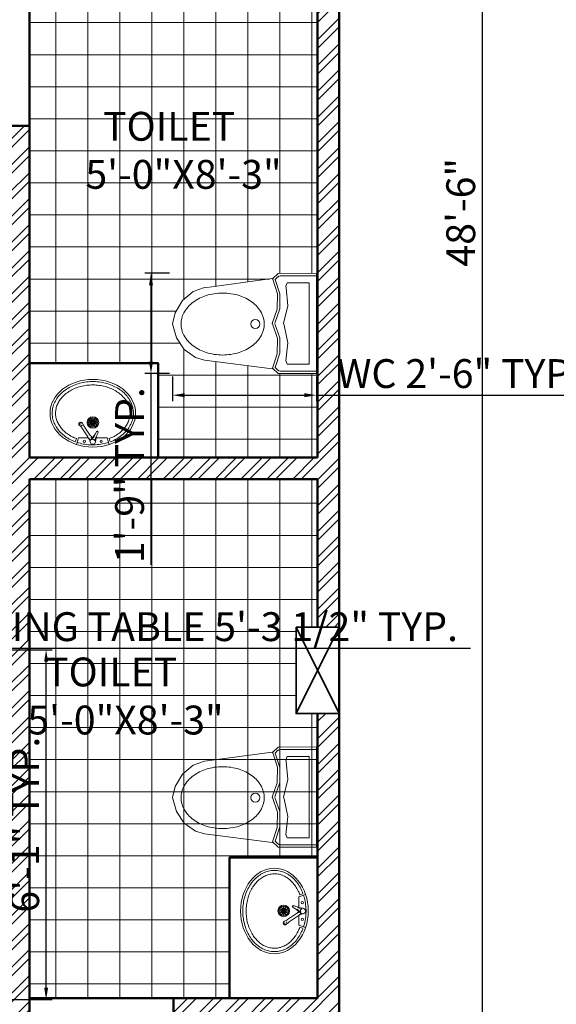
# Model space of a CAD drawing. Units: millimetres. Extents: x 67033 to 68301, y 155969 to 157209.
# Tile 13 of 17: x 67771 to 67883, y 156689 to 156894. Entities that reach past the tile are written whole.
import ezdxf

# ---------------------------------------------------------------- set-up
doc = ezdxf.new("R2010")
doc.units = ezdxf.units.MM
for name, color, linetype, lineweight in [('A-ANNO-DIMS', 2, 'Continuous', 18), ('A-AREA-IDEN', 3, 'Continuous', 18), ('A-COLS', 3, 'Continuous', 35), ('A-FLOR-FIXT', 9, 'Continuous', 18), ('A-FLOR-PATT', 252, 'Continuous', 13), ('A-WALL', 7, 'Continuous', 50), ('A-WALL-PATT', 8, 'Continuous', 13)]:
    doc.layers.add(name, color=color, linetype=linetype, lineweight=lineweight)
doc.styles.get("Standard").update_dxf_attribs({"font": 'arial.ttf'})
doc.dimstyles.new('ISO-25', dxfattribs={"dimtxt": 6, "dimasz": 2.5, "dimexe": 1.25, "dimexo": 0.625, "dimtad": 1, "dimdec": 0, "dimlunit": 3, "dimtxsty": 'Standard', "dimcen": 2.5, "dimadec": 0, "dimazin": 0, "dimtfac": 1, "dimtdec": 0, "dimtmove": 0, "dimatfit": 3, "dimfxl": 1, "dimarcsym": 0})
pattern_1 = [(45, (429.8785, 0), (-2.69407684, 2.69407684), []), (45, (431.6745, 0), (-2.69407684, 2.69407684), [])]
pattern_2 = [(0, (429.8785, 0), (0, 6.6675), []), (90, (429.8785, 0), (-6.6675, 4e-16), [])]

# ---------------------------------------------------------------- blocks, each defined once
blk = doc.blocks.new('A$C1AC47749')
for p, q in [((0.1857, 0.4482), (0.192, 0.4291)), ((0.1907, 0.471), (0.2068, 0.4222)), ((0.4293, 0.471), (0.4132, 0.4222)), ((0.4343, 0.4482), (0.428, 0.4291)), ((0.2068, 0.4222), (0.2842, 0.4222)), ((0.328, 0.4053), (0.3724, 0.3403)), ((0.4132, 0.4222), (0.3413, 0.4222)), ((0.3893, 0.3519), (0.3454, 0.4162))]:
    blk.add_line(p, q)
for centre, radius in [((0.2494, 0.448), 0.00831), ((0.3706, 0.448), 0.00831), ((0.3092, 0.3122), 0.0419), ((0.3092, 0.3122), 0.0344), ((0.3092, 0.3122), 0.00537)]:
    blk.add_circle(centre, radius)
for centre, radius, start, end in [((0.0375, 0.4868), 0.255, 336.13579, 352.27707), ((0.5085, 0.2596), 0.255, 136.21432, 152.3556), ((0.2063, 0.4499), 0.0866, 334.5047, 356.00596), ((0.31, 0.4499), 0.02, 316.21432, 172.27707), ((0.3092, 0.4498), 0.0162, 192.84427, 306.07085), ((0.3746, 0.3688), 0.0866, 132.48544, 153.98669), ((0.4278, 0.4728), 0.1, 191.02619, 214.5133), ((0.3603, 0.4414), 0.0293, 186.64626, 215.15328), ((0.2768, 0.381), 0.00664, 156.13579, 332.3556), ((0.2783, 0.3821), 0.00491, 187.76508, 270.74833), ((0.1778, 0.1242), 0.3257, 64.69826, 65.8021), ((0.2456, 0.3486), 0.1, 34.51324, 47.88111), ((0.299, 0.3998), 0.0293, 33.00691, 56.74915), ((0.29, 0.2836), 0.1, 20.01079, 34.51324), ((0.3971, 0.3226), 0.0139, 200.01079, 49.01574), ((0.3943, 0.3268), 0.00759, 93.32422, 152.57703), ((0.4717, 0.4086), 0.1, 214.5133, 229.01574), ((0.397, 0.323), 0.00812, 242.55567, 44.63645), ((0.3988, 0.322), 0.00965, 313.38275, 23.63796)]:
    blk.add_arc(centre, radius, start, end)
for centre, major_axis, ratio in [((0.31, 0.2449), (-0.31, 0), 0.790323), ((0.2894, 0.3122), (0.0145, 0), 0.137964), ((0.292, 0.3221), (0.0126, -0.0072), 0.137964), ((0.292, 0.3022), (0.0126, 0.0072), 0.137964), ((0.2993, 0.3294), (0.0072, -0.0126), 0.137964), ((0.2993, 0.295), (0.0072, 0.0126), 0.137964), ((0.3092, 0.332), (0, -0.0145), 0.137964), ((0.3092, 0.2923), (0, 0.0145), 0.137964), ((0.3192, 0.3294), (-0.0072, -0.0126), 0.137964), ((0.3192, 0.295), (-0.0072, 0.0126), 0.137964), ((0.3264, 0.3221), (-0.0126, -0.0072), 0.137964), ((0.3264, 0.3022), (-0.0126, 0.0072), 0.137964), ((0.3291, 0.3122), (-0.0145, 0), 0.137964)]:
    blk.add_ellipse(centre, major_axis=major_axis, ratio=ratio)
for points, knots in [([(0.1844, 0.4522), (0.1793, 0.4504), (0.1743, 0.4484), (0.1546, 0.44), (0.1406, 0.4328), (0.1143, 0.4165), (0.102, 0.4076), (0.0797, 0.3882), (0.0697, 0.3778), (0.052, 0.3558), (0.0443, 0.3443), (0.0317, 0.3205), (0.0267, 0.3083), (0.0194, 0.2833), (0.0171, 0.2706), (0.0158, 0.2536), (0.0156, 0.2492), (0.0156, 0.2449), (0.0156, 0.2369), (0.0162, 0.229), (0.019, 0.2084), (0.022, 0.1958), (0.0309, 0.1711), (0.0366, 0.159), (0.0508, 0.1357), (0.0591, 0.1244), (0.0781, 0.1031), (0.0888, 0.0931), (0.1123, 0.0746), (0.1251, 0.066), (0.1524, 0.0508), (0.1669, 0.0441), (0.1972, 0.0327), (0.213, 0.028), (0.2454, 0.0207), (0.262, 0.0182), (0.2956, 0.0154), (0.3125, 0.0152), (0.3462, 0.0169), (0.3629, 0.0189), (0.3956, 0.0251), (0.4117, 0.0293), (0.4426, 0.0397), (0.4574, 0.046), (0.4855, 0.0604), (0.4987, 0.0685), (0.5232, 0.0863), (0.5344, 0.096), (0.5545, 0.1167), (0.5635, 0.1277), (0.5788, 0.1506), (0.5851, 0.1625), (0.5953, 0.187), (0.599, 0.1995), (0.6037, 0.2248), (0.6047, 0.2375), (0.6039, 0.263), (0.6021, 0.2758), (0.5959, 0.3009), (0.5914, 0.3133), (0.5798, 0.3373), (0.5727, 0.349), (0.556, 0.3714), (0.5464, 0.382), (0.5249, 0.402), (0.5131, 0.4113), (0.4875, 0.4282), (0.4738, 0.4358), (0.4516, 0.446), (0.4437, 0.4492), (0.4356, 0.4522)], [5.14883, 5.14883, 5.14883, 5.14883, 5.205467, 5.205467, 5.375452, 5.375452, 5.545437, 5.545437, 5.715422, 5.715422, 5.885408, 5.885408, 6.055393, 6.055393, 6.225378, 6.225378, 6.283185, 6.283185, 6.283185, 6.389094, 6.389094, 6.559079, 6.559079, 6.729064, 6.729064, 6.89905, 6.89905, 7.069035, 7.069035, 7.23902, 7.23902, 7.409005, 7.409005, 7.578991, 7.578991, 7.748976, 7.748976, 7.918961, 7.918961, 8.088947, 8.088947, 8.258932, 8.258932, 8.428917, 8.428917, 8.598902, 8.598902, 8.768888, 8.768888, 8.938873, 8.938873, 9.108858, 9.108858, 9.278843, 9.278843, 9.448829, 9.448829, 9.618814, 9.618814, 9.788799, 9.788799, 9.958784, 9.958784, 10.12877, 10.12877, 10.298755, 10.298755, 10.46874, 10.46874, 10.559126, 10.559126, 10.559126, 10.559126]), ([(0.192, 0.4291), (0.1828, 0.4257), (0.1739, 0.4219), (0.1529, 0.4117), (0.1412, 0.4049), (0.1193, 0.3901), (0.1093, 0.382), (0.0911, 0.3649), (0.0829, 0.3558), (0.0687, 0.3371), (0.0626, 0.3273), (0.0526, 0.3074), (0.0487, 0.2972), (0.043, 0.2767), (0.0411, 0.2663), (0.0401, 0.2522), (0.04, 0.2486), (0.04, 0.2449), (0.04, 0.2369), (0.0406, 0.229), (0.0435, 0.2107), (0.0461, 0.2004), (0.0536, 0.1801), (0.0584, 0.1701), (0.0702, 0.1506), (0.0771, 0.1411), (0.093, 0.1229), (0.1019, 0.1142), (0.1217, 0.098), (0.1324, 0.0904), (0.1556, 0.0766), (0.168, 0.0704), (0.1939, 0.0596), (0.2075, 0.055), (0.2356, 0.0476), (0.2501, 0.0447), (0.2794, 0.0409), (0.2943, 0.0399), (0.3242, 0.0398), (0.3391, 0.0408), (0.3685, 0.0445), (0.3829, 0.0472), (0.4111, 0.0546), (0.4247, 0.0591), (0.4508, 0.0698), (0.4632, 0.076), (0.4864, 0.0897), (0.4973, 0.0972), (0.5171, 0.1134), (0.5262, 0.122), (0.5422, 0.1401), (0.5492, 0.1496), (0.561, 0.1691), (0.5659, 0.1791), (0.5736, 0.1994), (0.5763, 0.2097), (0.5797, 0.2304), (0.5803, 0.2408), (0.5794, 0.2617), (0.5779, 0.272), (0.5728, 0.2926), (0.5692, 0.3029), (0.5599, 0.3229), (0.5541, 0.3327), (0.5405, 0.3517), (0.5327, 0.3609), (0.5151, 0.3783), (0.5053, 0.3865), (0.4839, 0.4017), (0.4724, 0.4087), (0.4499, 0.4202), (0.4392, 0.4249), (0.428, 0.4291)], [5.15203, 5.15203, 5.15203, 5.15203, 5.262547, 5.262547, 5.423175, 5.423175, 5.583803, 5.583803, 5.744431, 5.744431, 5.90506, 5.90506, 6.065688, 6.065688, 6.226316, 6.226316, 6.283185, 6.283185, 6.283185, 6.405631, 6.405631, 6.566259, 6.566259, 6.726887, 6.726887, 6.887515, 6.887515, 7.048143, 7.048143, 7.208772, 7.208772, 7.3694, 7.3694, 7.530028, 7.530028, 7.690656, 7.690656, 7.851284, 7.851284, 8.011912, 8.011912, 8.172541, 8.172541, 8.333169, 8.333169, 8.493797, 8.493797, 8.654425, 8.654425, 8.815053, 8.815053, 8.975681, 8.975681, 9.13631, 9.13631, 9.296938, 9.296938, 9.457566, 9.457566, 9.618194, 9.618194, 9.778822, 9.778822, 9.93945, 9.93945, 10.100079, 10.100079, 10.260707, 10.260707, 10.421335, 10.421335, 10.555929, 10.555929, 10.555929, 10.555929]), ([(0.4244, 0.4561), (0.4209, 0.4573), (0.4174, 0.4584), (0.3981, 0.4641), (0.3818, 0.4677), (0.3487, 0.4726), (0.3319, 0.474), (0.2982, 0.4744), (0.2813, 0.4735), (0.248, 0.4694), (0.2315, 0.4663), (0.2088, 0.4603), (0.2022, 0.4583), (0.1956, 0.4561)], [4.3173628, 4.3173628, 4.3173628, 4.3173628, 4.3555402, 4.3555402, 4.5255255, 4.5255255, 4.6955107, 4.6955107, 4.865496, 4.865496, 5.0354813, 5.0354813, 5.1074083, 5.1074083, 5.1074083, 5.1074083])]:
    blk.add_open_spline(points, degree=3, knots=knots)
blk = doc.blocks.new('A$C09D638C3')
for p, q in [((0, 0.7166), (0.0008, 0.5263)), ((0.2504, 0.7166), (0, 0.7166)), ((0.0137, 0.7166), (0.0137, 0.5365)), ((0.2504, 0.7166), (0.5, 0.7166)), ((0.4871, 0.7166), (0.4871, 0.5365)), ((0.5, 0.7166), (0.5, 0.5263)), ((0.048, 0.6794), (0.048, 0.5712)), ((0.2504, 0.6794), (0.048, 0.6794)), ((0.2504, 0.6794), (0.4528, 0.6794)), ((0.4528, 0.6794), (0.4528, 0.5712)), ((0.048, 0.5712), (0.0652, 0.5632)), ((0.0733, 0.5655), (0.0652, 0.5632)), ((0.1631, 0.5735), (0.0733, 0.5655)), ((0.2504, 0.5527), (0.1631, 0.5735)), ((0.2582, 0.5558), (0.2504, 0.5527)), ((0.3462, 0.574), (0.2582, 0.5558)), ((0.4356, 0.5632), (0.3462, 0.574)), ((0.4528, 0.5712), (0.4356, 0.5632)), ((0.0008, 0.5263), (0.0274, 0.4973)), ((0.0137, 0.5365), (0.015, 0.5295)), ((0.015, 0.5295), (0.0189, 0.5233)), ((0.0189, 0.5233), (0.019, 0.5232)), ((0.019, 0.5232), (0.0309, 0.5105)), ((0.0271, 0.4967), (0.072, 0.1582)), ((0.0297, 0.4985), (0.0274, 0.4973)), ((0.102, 0.522), (0.0297, 0.4985)), ((0.1021, 0.5341), (0.0309, 0.5105)), ((0.1786, 0.5213), (0.102, 0.522)), ((0.1781, 0.5339), (0.1021, 0.5341)), ((0.2494, 0.5098), (0.1781, 0.5339)), ((0.2504, 0.4965), (0.1786, 0.5213)), ((0.2527, 0.4977), (0.2504, 0.4965)), ((0.3224, 0.5339), (0.2514, 0.5098)), ((0.3248, 0.5217), (0.2527, 0.4977)), ((0.3984, 0.5342), (0.3224, 0.5339)), ((0.4014, 0.5216), (0.3248, 0.5217)), ((0.47, 0.5105), (0.3984, 0.5342)), ((0.4734, 0.4973), (0.4014, 0.5216)), ((0.4758, 0.4967), (0.4334, 0.1581)), ((0.4818, 0.5232), (0.47, 0.5105)), ((0.5, 0.5263), (0.4734, 0.4973)), ((0.4818, 0.5232), (0.4857, 0.5293)), ((0.4857, 0.5293), (0.4871, 0.5363)), ((0.4871, 0.5363), (0.4871, 0.5365)), ((0.0718, 0.1596), (0.0917, 0.1021)), ((0.4201, 0.1144), (0.4334, 0.1581)), ((0.0917, 0.1021), (0.1359, 0.0488)), ((0.3799, 0.0583), (0.4201, 0.1144)), ((0.3218, 0.0186), (0.3799, 0.0583)), ((0.1359, 0.0488), (0.1968, 0.0131)), ((0.1968, 0.0131), (0.2526, 0)), ((0.2528, 0), (0.3218, 0.0186))]:
    blk.add_line(p, q)
blk.add_circle((0.2527, 0.4124), 0.0222)
for centre, radius, start, end in [((0.2776, 0.2962), 0.1668, 118.8748, 143.2661), ((0.2513, 0.3471), 0.1095, 89.1493, 119.7298), ((0.2546, 0.3471), 0.1095, 60.2702, 90.8507), ((0.2283, 0.2962), 0.1668, 36.7339, 61.1252), ((0.3216, 0.265), 0.2207, 143.6094, 162.4475), ((0.1843, 0.265), 0.2207, 17.5525, 36.3906), ((0.3937, 0.2468), 0.295, 163.3175, 179.5076), ((0.1122, 0.2468), 0.295, 0.4924, 16.6825), ((0.3937, 0.2519), 0.295, 180.4924, 196.6825), ((0.1122, 0.2519), 0.295, 343.3175, 359.5076), ((0.3216, 0.2338), 0.2207, 197.5525, 216.3906), ((0.1843, 0.2338), 0.2207, 323.6094, 342.4475), ((0.2776, 0.2026), 0.1668, 216.7339, 241.1252), ((0.2283, 0.2026), 0.1668, 298.8748, 323.2661), ((0.2513, 0.1516), 0.1095, 240.2702, 270.8507), ((0.2546, 0.1516), 0.1095, 269.1493, 299.7298)]:
    blk.add_arc(centre, radius, start, end)
blk = doc.blocks.new('COLUMN-230x460')
for p, q in [((0.44, 17.99), (9.44, -0.01)), ((9.44, 17.99), (0.44, -0.01))]:
    blk.add_line(p, q)
blk.add_lwpolyline([(0.44, 17.99), (9.44, 17.99), (9.44, -0.01), (0.44, -0.01)], close=True)
blk = doc.blocks.new('*D57')
at = {"layer": 'A-ANNO-DIMS', "color": 0, "lineweight": -2, "transparency": 16777216}
for p, q in [((67675.78, 156689.05), (67675.78, 156675.31)), ((67763.19, 156689.05), (67763.19, 156675.31)), ((67678.28, 156676.56), (67760.69, 156676.56)), ((67763.19, 156676.56), (67873.56, 156676.56))]:
    blk.add_line(p, q, dxfattribs=at)
at = {"layer": 'A-ANNO-DIMS', "color": 0, "transparency": 16777216}
for points in [[(67678.28, 156676.98), (67678.28, 156676.14), (67675.78, 156676.56)], [(67760.69, 156676.98), (67760.69, 156676.14), (67763.19, 156676.56)]]:
    blk.add_solid(points, dxfattribs=at)
at = {"layer": 'Defpoints', "color": 0, "transparency": 16777216}
for p in [(67675.78, 156689.67), (67763.19, 156689.67), (67763.19, 156676.56)]:
    blk.add_point(p, dxfattribs=at)
at = {"layer": 'A-ANNO-DIMS', "color": 0, "transparency": 16777216, "insert": (67819.62, 156680.29), "char_height": 6, "attachment_point": 5}
blk.add_mtext('DOUBLE BED 7\'-3 1/2" TYP.', dxfattribs=at)
blk = doc.blocks.new('*D58')
at = {"layer": 'A-ANNO-DIMS', "color": 0, "lineweight": -2, "transparency": 16777216}
for p, q in [((67763.82, 156762.48), (67777.55, 156762.48)), ((67776.3, 156692.17), (67776.3, 156759.98)), ((67763.82, 156689.67), (67777.55, 156689.67))]:
    blk.add_line(p, q, dxfattribs=at)
at = {"layer": 'A-ANNO-DIMS', "color": 0, "transparency": 16777216}
for points in [[(67775.89, 156759.98), (67776.72, 156759.98), (67776.3, 156762.48)], [(67775.89, 156692.17), (67776.72, 156692.17), (67776.3, 156689.67)]]:
    blk.add_solid(points, dxfattribs=at)
at = {"layer": 'Defpoints', "color": 0, "transparency": 16777216}
for p in [(67763.19, 156762.48), (67776.3, 156762.48), (67763.19, 156689.67)]:
    blk.add_point(p, dxfattribs=at)
at = {"layer": 'A-ANNO-DIMS', "color": 0, "transparency": 16777216, "insert": (67772.62, 156726.07), "char_height": 6, "attachment_point": 5, "rotation": 90}
blk.add_mtext('6\'-1" TYP.', dxfattribs=at)
blk = doc.blocks.new('*D59')
at = {"layer": 'A-ANNO-DIMS', "color": 0, "lineweight": -2, "transparency": 16777216}
for p, q in [((67802.63, 156819.29), (67802.63, 156814.18)), ((67832.57, 156819.29), (67832.57, 156814.18)), ((67805.13, 156815.43), (67830.07, 156815.43)), ((67832.57, 156815.43), (67889.44, 156815.43))]:
    blk.add_line(p, q, dxfattribs=at)
at = {"layer": 'A-ANNO-DIMS', "color": 0, "transparency": 16777216}
for points in [[(67805.13, 156815.84), (67805.13, 156815.01), (67802.63, 156815.43)], [(67830.07, 156815.84), (67830.07, 156815.01), (67832.57, 156815.43)]]:
    blk.add_solid(points, dxfattribs=at)
at = {"layer": 'Defpoints', "color": 0, "transparency": 16777216}
for p in [(67802.63, 156819.92), (67832.57, 156819.92), (67832.57, 156815.43)]:
    blk.add_point(p, dxfattribs=at)
at = {"layer": 'A-ANNO-DIMS', "color": 0, "transparency": 16777216, "insert": (67862.26, 156819.15), "char_height": 6, "attachment_point": 5}
blk.add_mtext('WC 2\'-6" TYP.', dxfattribs=at)
blk = doc.blocks.new('*D60')
at = {"layer": 'A-ANNO-DIMS', "color": 0, "lineweight": -2, "transparency": 16777216}
for p, q in [((67802, 156840.81), (67796.88, 156840.81)), ((67798.13, 156838.31), (67798.13, 156822.42)), ((67802, 156819.92), (67796.88, 156819.92)), ((67798.13, 156819.92), (67798.13, 156780.16))]:
    blk.add_line(p, q, dxfattribs=at)
at = {"layer": 'A-ANNO-DIMS', "color": 0, "transparency": 16777216}
for points in [[(67797.72, 156838.31), (67798.55, 156838.31), (67798.13, 156840.81)], [(67797.72, 156822.42), (67798.55, 156822.42), (67798.13, 156819.92)]]:
    blk.add_solid(points, dxfattribs=at)
at = {"layer": 'Defpoints', "color": 0, "transparency": 16777216}
for p in [(67802.63, 156840.81), (67798.13, 156819.92), (67802.63, 156819.92)]:
    blk.add_point(p, dxfattribs=at)
at = {"layer": 'A-ANNO-DIMS', "color": 0, "transparency": 16777216, "insert": (67794.45, 156798.79), "char_height": 6, "attachment_point": 5, "rotation": 90}
blk.add_mtext('1\'-9" TYP.', dxfattribs=at)
blk = doc.blocks.new('*D67')
at = {"layer": 'A-ANNO-DIMS', "color": 0, "lineweight": -2, "transparency": 16777216}
for p, q in [((67686.77, 156771.63), (67686.77, 156761.51)), ((67750.09, 156771.63), (67750.09, 156761.51)), ((67689.27, 156762.76), (67747.59, 156762.76)), ((67750.09, 156762.76), (67864.65, 156762.76))]:
    blk.add_line(p, q, dxfattribs=at)
at = {"layer": 'A-ANNO-DIMS', "color": 0, "transparency": 16777216}
for points in [[(67689.27, 156763.18), (67689.27, 156762.34), (67686.77, 156762.76)], [(67747.59, 156763.18), (67747.59, 156762.34), (67750.09, 156762.76)]]:
    blk.add_solid(points, dxfattribs=at)
at = {"layer": 'Defpoints', "color": 0, "transparency": 16777216}
for p in [(67686.77, 156772.26), (67750.09, 156772.26), (67750.09, 156762.76)]:
    blk.add_point(p, dxfattribs=at)
at = {"layer": 'A-ANNO-DIMS', "color": 0, "transparency": 16777216, "insert": (67808.62, 156766.49), "char_height": 6, "attachment_point": 5}
blk.add_mtext('DINING TABLE 5\'-3 1/2" TYP.', dxfattribs=at)
blk = doc.blocks.new('*D112')
at = {"layer": 'A-ANNO-DIMS', "color": 0, "lineweight": -2, "transparency": 16777216}
for p, q in [((67601.44, 157144.49), (67868.32, 157144.49)), ((67867.07, 157141.99), (67867.07, 156564.99)), ((67768.94, 156562.49), (67868.32, 156562.49))]:
    blk.add_line(p, q, dxfattribs=at)
at = {"layer": 'A-ANNO-DIMS', "color": 0, "transparency": 16777216}
for points in [[(67866.65, 157141.99), (67867.48, 157141.99), (67867.07, 157144.49)], [(67866.65, 156564.99), (67867.48, 156564.99), (67867.07, 156562.49)]]:
    blk.add_solid(points, dxfattribs=at)
at = {"layer": 'Defpoints', "color": 0, "transparency": 16777216}
for p in [(67600.82, 157144.49), (67768.32, 156562.49), (67867.07, 156562.49)]:
    blk.add_point(p, dxfattribs=at)
at = {"layer": 'A-ANNO-DIMS', "color": 0, "transparency": 16777216, "insert": (67863.38, 156853.49), "char_height": 6, "attachment_point": 5, "rotation": 90}
blk.add_mtext('48\'-6"', dxfattribs=at)

msp = doc.modelspace()

# ---------------------------------------------------------------- hatches: boundary and pattern name
at = {"layer": 'A-FLOR-PATT'}
h = msp.add_hatch(dxfattribs=at)
h.set_pattern_fill('NET', color=256, scale=2.1)
h.set_pattern_definition(pattern_2)
h.paths.add_polyline_path([(67832.82, 156901.49), (67820.82, 156901.49), (67820.82, 156905.99), (67790.82, 156905.99), (67790.82, 156901.49), (67772.82, 156901.49), (67772.82, 156871.49), (67772.82, 156822.09), (67799.66, 156822.09), (67799.66, 156802.49), (67832.82, 156802.49)])
h.paths.add_polyline_path([(67823.43, 156839.69), (67824.62, 156840.78), (67832.57, 156840.81), (67832.57, 156830.35), (67832.57, 156819.92), (67824.62, 156819.92), (67823.54, 156820.91), (67809.23, 156822.7), (67807.41, 156823.26), (67805.06, 156824.94), (67803.4, 156827.36), (67802.63, 156830.25), (67803.17, 156832.59), (67804.67, 156835.13), (67806.89, 156836.98), (67809.3, 156837.81)], flags=16)
h.paths.add_polyline_path([(67813.05, 156836.69, -0.07076), (67816.48, 156836.17, -0.082382), (67819.17, 156834.8, -0.106831), (67821.11, 156832.58, -0.13423), (67821.71, 156830.24, -0.13423), (67821.11, 156827.91, -0.106831), (67819.17, 156825.68, -0.082382), (67816.48, 156824.32, -0.07076), (67813.05, 156823.8, -0.07076), (67809.61, 156824.32, -0.082382), (67806.92, 156825.68, -0.106831), (67804.99, 156827.91, -0.13423), (67804.39, 156830.24, -0.13423), (67804.99, 156832.58, -0.106831), (67806.92, 156834.8, -0.082382), (67809.61, 156836.17, -0.07076)], flags=0)
h.paths.add_polyline_path([(67823.39, 156830.38), (67823.43, 156830.25), (67823.38, 156830.35)], flags=0)
h.paths.add_polyline_path([(67824.5, 156840.03), (67824.49, 156840.02), (67823.96, 156839.53), (67824.95, 156836.55), (67824.94, 156833.37), (67823.92, 156830.35), (67824.94, 156827.34), (67824.95, 156824.16), (67823.96, 156821.17), (67824.49, 156820.68), (67824.75, 156820.52), (67825.04, 156820.46), (67825.05, 156820.46), (67825.04, 156820.46), (67824.75, 156820.52), (67824.49, 156820.68), (67823.96, 156821.17), (67824.95, 156824.16), (67824.94, 156827.34), (67823.92, 156830.35), (67824.94, 156833.37), (67824.95, 156836.55), (67823.96, 156839.53), (67824.5, 156840.03)], flags=0)
h.paths.add_polyline_path([(67826.5, 156838.81), (67831.02, 156838.81), (67831.02, 156830.35), (67831.02, 156821.89), (67826.5, 156821.89), (67826.17, 156822.61), (67826.61, 156826.35), (67825.85, 156830.02), (67825.72, 156830.35), (67826.59, 156834), (67826.26, 156837.75), (67826.17, 156838.09)], flags=0)
h.paths.add_polyline_path([(67820.79, 156830.25, -1), (67818.94, 156830.25, -1)], flags=0)
h.paths.add_polyline_path([(67792.51, 156895.05), (67814.14, 156895.05), (67814.14, 156907.42), (67792.51, 156907.42)], flags=9)
h.paths.add_polyline_path([(67782.63, 156854.97), (67824.6, 156854.97), (67824.6, 156877.36), (67782.63, 156877.36)], flags=24)
h = msp.add_hatch(dxfattribs=at)
h.set_pattern_fill('NET', color=256, scale=2.1)
h.set_pattern_definition(pattern_2)
h.paths.add_polyline_path([(67832.82, 156797.99), (67772.82, 156797.99), (67772.82, 156689.99), (67802.82, 156689.99), (67814.5, 156689.99), (67814.5, 156719.26), (67832.82, 156719.26), (67832.82, 156749.19), (67828.32, 156749.19), (67828.32, 156767.19), (67832.82, 156767.19)])
h.paths.add_polyline_path([(67823.43, 156741.13), (67824.62, 156742.23), (67832.57, 156742.26), (67832.57, 156731.79), (67832.57, 156721.36), (67824.62, 156721.36), (67823.54, 156722.36), (67809.23, 156724.15), (67807.41, 156724.7), (67805.06, 156726.38), (67803.4, 156728.81), (67802.63, 156731.7), (67803.17, 156734.03), (67804.67, 156736.58), (67806.89, 156738.43), (67809.3, 156739.26)], flags=16)
h.paths.add_polyline_path([(67813.05, 156738.13, -0.07076), (67816.48, 156737.62, -0.082382), (67819.17, 156736.25, -0.106831), (67821.11, 156734.03, -0.13423), (67821.71, 156731.69, -0.13423), (67821.11, 156729.35, -0.106831), (67819.17, 156727.13, -0.082382), (67816.48, 156725.76, -0.07076), (67813.05, 156725.24, -0.07076), (67809.61, 156725.76, -0.082382), (67806.92, 156727.13, -0.106831), (67804.99, 156729.35, -0.13423), (67804.39, 156731.69, -0.13423), (67804.99, 156734.03, -0.106831), (67806.92, 156736.25, -0.082382), (67809.61, 156737.62, -0.07076)], flags=0)
h.paths.add_polyline_path([(67823.39, 156731.82), (67823.43, 156731.7), (67823.38, 156731.79)], flags=0)
h.paths.add_polyline_path([(67824.76, 156741.63), (67824.5, 156741.47), (67824.49, 156741.46), (67823.96, 156740.97), (67824.95, 156737.99), (67824.94, 156734.82), (67823.92, 156731.79), (67824.94, 156728.78), (67824.95, 156725.61), (67823.96, 156722.62), (67824.49, 156722.12), (67824.75, 156721.96), (67825.04, 156721.9), (67825.05, 156721.9), (67824.84, 156721.9), (67824.49, 156722.12), (67823.96, 156722.62), (67824.95, 156725.61), (67824.94, 156728.78), (67823.92, 156731.79), (67824.94, 156734.82), (67824.95, 156737.99), (67823.96, 156740.97), (67824.65, 156741.61)], flags=0)
h.paths.add_polyline_path([(67826.5, 156740.25), (67831.02, 156740.25), (67831.02, 156731.79), (67831.02, 156723.34), (67826.5, 156723.34), (67826.17, 156724.05), (67826.61, 156727.79), (67825.85, 156731.47), (67825.72, 156731.79), (67826.59, 156735.44), (67826.26, 156739.2), (67826.17, 156739.54)], flags=0)
h.paths.add_polyline_path([(67820.79, 156731.7, -1), (67818.94, 156731.7, -1)], flags=0)
h = msp.add_hatch(dxfattribs=at)
h.set_pattern_fill('NET', color=256, scale=2.1)
h.set_pattern_definition(pattern_2)
h.paths.add_polyline_path([(67823.43, 156741.13), (67824.62, 156742.23), (67832.57, 156742.26), (67832.57, 156731.79), (67832.57, 156721.36), (67824.62, 156721.36), (67823.54, 156722.36), (67809.23, 156724.15), (67807.41, 156724.7), (67805.06, 156726.38), (67803.4, 156728.81), (67802.63, 156731.7), (67803.17, 156734.03), (67804.67, 156736.58), (67806.89, 156738.43), (67809.3, 156739.26)], flags=16)
h.paths.add_polyline_path([(67759.9, 156741.43), (67815.84, 156741.43), (67815.84, 156763.82), (67759.9, 156763.82)], flags=9)
at = {"layer": 'A-WALL-PATT'}
h = msp.add_hatch(dxfattribs=at)
h.set_pattern_fill('ANSI32', color=256, scale=0.4)
h.set_pattern_definition(pattern_1)
h.paths.add_polyline_path([(67837.32, 156941.99), (67832.82, 156941.99), (67832.82, 156802.49), (67772.82, 156802.49), (67772.82, 156822.09), (67772.82, 156871.49), (67768.32, 156871.49), (67768.32, 156770.99), (67666.32, 156770.99), (67666.32, 156766.49), (67768.32, 156766.49), (67768.32, 156685.49), (67772.82, 156685.49), (67772.82, 156797.99), (67832.82, 156797.99), (67832.82, 156767.19), (67837.32, 156767.19)])
h = msp.add_hatch(dxfattribs=at)
h.set_pattern_fill('ANSI32', color=256, scale=0.4)
h.set_pattern_definition(pattern_1)
h.paths.add_polyline_path([(67837.32, 156749.19), (67832.82, 156749.19), (67832.82, 156689.99), (67814.5, 156689.99), (67802.82, 156689.99), (67802.82, 156685.49), (67832.82, 156685.49), (67832.82, 156640.49), (67837.32, 156640.49)])

# ---------------------------------------------------------------- linework, layer by layer
at = {"layer": 'A-WALL'}
for p, q in [((67837.32, 157082.99), (67837.32, 156572.08)), ((67832.82, 156941.99), (67832.82, 156802.49)), ((67772.82, 156871.49), (67772.82, 156901.49)), ((67768.32, 156871.49), (67772.82, 156871.49)), ((67772.82, 156871.49), (67772.82, 156802.49)), ((67772.82, 156802.49), (67832.82, 156802.49)), ((67772.82, 156797.99), (67772.82, 156685.49)), ((67772.82, 156797.99), (67832.82, 156797.99)), ((67832.82, 156797.99), (67832.82, 156767.19)), ((67832.82, 156749.19), (67832.82, 156689.99)), ((67802.82, 156689.99), (67772.82, 156689.99)), ((67802.82, 156689.99), (67802.82, 156685.49)), ((67802.82, 156689.99), (67832.82, 156689.99))]:
    msp.add_line(p, q, dxfattribs=at)
for points in [[(67772.82, 156822.09), (67799.66, 156822.09), (67799.66, 156802.49), (67772.82, 156802.49)], [(67832.82, 156719.26), (67814.5, 156719.26), (67814.5, 156689.99), (67832.82, 156689.99)]]:
    msp.add_lwpolyline(points, close=True, dxfattribs=at)

# ---------------------------------------------------------------- block references
at = {"layer": 'A-COLS'}
msp.add_blockref('COLUMN-230x460', (67827.88, 156749.2), dxfattribs=at)
at = {"layer": 'A-FLOR-FIXT'}
for name, p, xscale, yscale, zscale, rotation in [('A$C09D638C3', (67802.63, 156840.81), 41.79230271587537, 41.79230271587537, 41.79230271587537, 270), ('A$C1AC47749', (67794.92, 156818.71), 28.71035709425095, 28.71035709425095, 28.71035709425095, 180), ('A$C09D638C3', (67802.63, 156742.26), 41.79230271587537, 41.79230271587537, 41.79230271587537, 270), ('A$C1AC47749', (67816.79, 156717), 28.71035709425095, 28.71035709425095, 28.71035709425095, 270)]:
    msp.add_blockref(name, p, dxfattribs=dict(at, xscale=xscale, yscale=yscale, zscale=zscale, rotation=rotation))

# ---------------------------------------------------------------- texts
at = {"layer": 'A-AREA-IDEN', "char_height": 6, "attachment_point": 1}
for s, width, insert in [('  TOILET                         5\'-0"X8\'-3"', 43.4182, (67784.47, 156874.38)), ('        TOILET\\P      5\'-0"X8\'-3"', 75.351, (67761.4, 156760.84))]:
    msp.add_mtext_dynamic_manual_height_columns(s, width=width, gutter_width=12.5, heights=[0], dxfattribs=dict(at, insert=insert))

# ---------------------------------------------------------------- dimensions: what is measured, and where the dimension line sits
at = {"layer": 'A-ANNO-DIMS'}
dim = msp.add_linear_dim(base=(67867.07, 156562.49), p1=(67600.82, 157144.49), p2=(67768.32, 156562.49), angle=90, dimstyle='ISO-25', override={"dimdec": 1, "dimlfac": 1, "dimrnd": 0, "dimzin": 1, "dimdsep": 46, "dimlunit": 4, "dimfrac": 2}, dxfattribs=at)
dim.commit()
dim.dimension.update_dxf_attribs({"geometry": '*D112', "text_midpoint": (67863.38, 156853.49)})
for base, p1, p2, angle, picture, middle in [((67798.13, 156819.92), (67802.63, 156840.81), (67802.63, 156819.92), 270, '*D60', (67794.45, 156798.79)), ((67776.3, 156762.48), (67763.19, 156689.67), (67763.19, 156762.48), 90, '*D58', (67772.62, 156726.07))]:
    dim = msp.add_linear_dim(base=base, p1=p1, p2=p2, angle=angle, text='<> TYP.', dimstyle='ISO-25', override={"dimdec": 1, "dimrnd": 0, "dimzin": 1, "dimlunit": 4, "dimfrac": 2}, dxfattribs=at)
    dim.commit()
    dim.dimension.update_dxf_attribs({"geometry": picture, "text_midpoint": middle})
for base, p1, p2, text, picture, middle in [((67832.57, 156815.43), (67802.63, 156819.92), (67832.57, 156819.92), 'WC <> TYP.', '*D59', (67862.26, 156819.15)), ((67750.09, 156762.76), (67686.77, 156772.26), (67750.09, 156772.26), 'DINING TABLE <> TYP.', '*D67', (67808.62, 156766.49)), ((67763.19, 156676.56), (67675.78, 156689.67), (67763.19, 156689.67), 'DOUBLE BED <> TYP.', '*D57', (67819.62, 156680.29))]:
    dim = msp.add_linear_dim(base=base, p1=p1, p2=p2, text=text, dimstyle='ISO-25', override={"dimdec": 1, "dimrnd": 0, "dimzin": 1, "dimlunit": 4, "dimfrac": 2}, dxfattribs=at)
    dim.commit()
    dim.dimension.update_dxf_attribs({"geometry": picture, "text_midpoint": middle})

doc.saveas('drawing.dxf')
